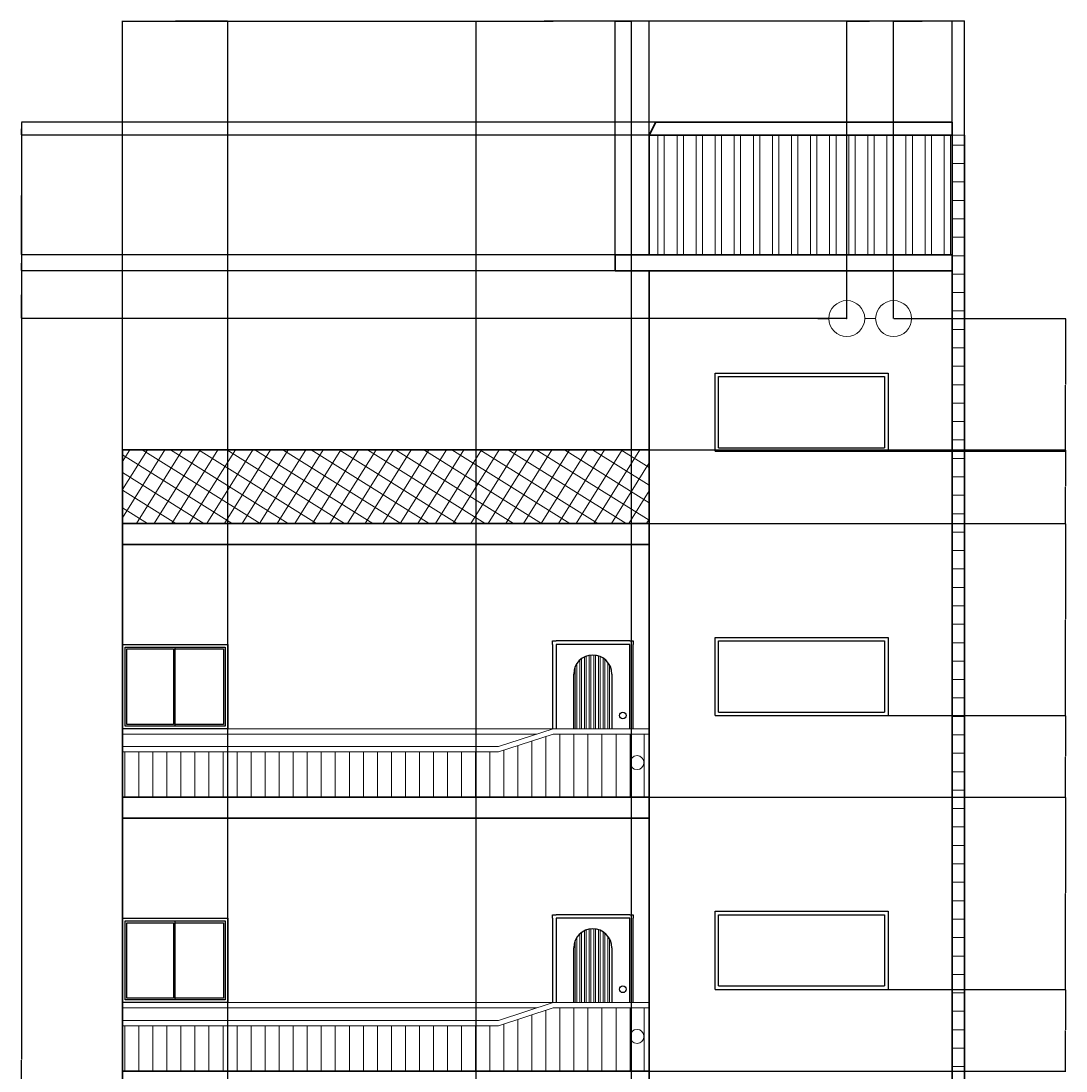
# Model space of a CAD drawing. Units: inches. Extents: x 373 to 969, y 157 to 1341.
# Tile 3 of 3: x 373 to 968, y 743 to 1341. Entities that reach past the tile are written whole.
import ezdxf

# ---------------------------------------------------------------- set-up
doc = ezdxf.new("R2010")
doc.units = ezdxf.units.IN
doc.header["$MEASUREMENT"] = 0
for name, color, linetype, lineweight in [('A-ANNO-DIMS', 2, 'Continuous', 18), ('A-DOOR', 3, 'Continuous', 25), ('A-DOOR-PATT', 8, 'Continuous', 13), ('A-ELEV-TRIM', 9, 'Continuous', 18), ('A-FLOR', 7, 'Continuous', 30), ('A-FLOR-HRAL', 4, 'Continuous', 18), ('A-FLOR-HRAL-PATT', 8, 'Continuous', 13), ('A-GLAZ', 4, 'Continuous', 25), ('A-ROOF', 7, 'Continuous', 30), ('A-WALL', 7, 'Continuous', 35), ('A-WALL-PATT', 8, 'Continuous', 13)]:
    doc.layers.add(name, color=color, linetype=linetype, lineweight=lineweight)
doc.styles.get("Standard").update_dxf_attribs({"font": 'arial.ttf'})
doc.dimstyles.get("Standard").update_dxf_attribs({"dimtxt": 0.18, "dimasz": 0.18, "dimexe": 0.18, "dimexo": 0.0625, "dimgap": 0.09, "dimtad": 0, "dimtih": 1, "dimtoh": 1, "dimdec": 4, "dimzin": 0, "dimdsep": 46, "dimlunit": 4, "dimtxsty": 'Standard', "dimcen": 0.09, "dimadec": 0, "dimazin": 0, "dimtfac": 1, "dimtdec": 4, "dimtofl": 0, "dimtmove": 0, "dimatfit": 3, "dimfxl": 1, "dimtolj": 1, "dimtzin": 0, "dimarcsym": 0})

# ---------------------------------------------------------------- blocks, each defined once
blk = doc.blocks.new('*U2')
for p, q in [((1.5, 1.5), (1.5, 46.5)), ((1.5, 46.5), (30, 46.5)), ((30, 1.5), (30, 46.5)), ((30, 46.5), (58.5, 46.5)), ((58.5, 46.5), (58.5, 1.5)), ((30, 1.5), (1.5, 1.5)), ((58.5, 1.5), (30, 1.5))]:
    blk.add_line(p, q)
blk.add_lwpolyline([(0, 0), (0, 48), (60, 48), (60, 0)], close=True)
for points in [[(29, 45.5), (29, 2.5), (2.5, 2.5), (2.5, 45.5), (29, 45.5)], [(30, 45.5), (57.5, 45.5), (57.5, 2.5), (30, 2.5)]]:
    blk.add_lwpolyline(points)
blk = doc.blocks.new('DOOR-ARCH-PANEL-ELEV')
for p, q in [((0, 48), (0, 50)), ((0, 50), (2, 50)), ((0, 48), (0, 0)), ((44, 50), (2, 50)), ((44, 48), (2, 48)), ((2, 48), (2, 0)), ((44, 50), (46, 50)), ((44, 0), (44, 48)), ((46, 50), (46, 48)), ((46, 0), (46, 48))]:
    blk.add_line(p, q)
for points in [[(12.07, 0), (12.07, 31.15)], [(33.78, 31.15), (33.78, 0)]]:
    blk.add_lwpolyline(points)
blk.add_circle((40.06, 7.56), 1.92)
blk.add_arc((22.93, 31.15), 10.86, 0, 180)
blk = doc.blocks.new('RAIL-BALCONY-SLOPED-ELEV')
for p, q in [((245.4, 23.26), (0, 23.26)), ((236.25, 20.26), (0, 20.26)), ((245.4, 23.26), (214.4, 13.09)), ((245.4, 20.26), (214.4, 10.09)), ((300.23, 23.26), (245.4, 23.26)), ((300.23, 20.26), (245.4, 20.26)), ((214.4, 13.09), (0, 13.09)), ((214.4, 10.09), (0, 10.09))]:
    blk.add_line(p, q)
blk.add_circle((293.27, 3.97), 3.97)
blk = doc.blocks.new('WIN-FIXED-FRAME-ELEV')
for p, q in [((0, 0), (98.59, 0)), ((2, 2), (96.59, 2))]:
    blk.add_line(p, q)
for points in [[(0, 0), (0, 44.5), (98.59, 44.5), (98.59, 0)], [(2, 2), (2, 42.5), (96.59, 42.5), (96.59, 2)]]:
    blk.add_lwpolyline(points)
blk = doc.blocks.new('*D20')
at = {"layer": 'A-ANNO-DIMS', "color": 0, "lineweight": -2, "transparency": 16777216}
for p, q in [((867.13, 789.48), (968.33, 789.48)), ((968.15, 789.3), (968.15, 766.42)), ((968.15, 743.16), (968.15, 766.05)), ((731, 742.98), (968.33, 742.98))]:
    blk.add_line(p, q, dxfattribs=at)
at = {"layer": 'A-ANNO-DIMS', "color": 0, "transparency": 16777216}
for points in [[(968.12, 789.3), (968.18, 789.3), (968.15, 789.48)], [(968.12, 743.16), (968.18, 743.16), (968.15, 742.98)]]:
    blk.add_solid(points, dxfattribs=at)
at = {"layer": 'Defpoints', "color": 0, "transparency": 16777216}
for p in [(867.07, 789.48), (968.15, 789.48), (730.93, 742.98)]:
    blk.add_point(p, dxfattribs=at)
at = {"layer": 'A-ANNO-DIMS', "color": 0, "transparency": 16777216, "insert": (968.15, 766.23), "char_height": 0.18, "attachment_point": 5}
blk.add_mtext('\\A1;46.5', dxfattribs=at)
blk = doc.blocks.new('*D21')
at = {"layer": 'A-ANNO-DIMS', "color": 0, "lineweight": -2, "transparency": 16777216}
for p, q in [((731, 898.98), (968.33, 898.98)), ((968.15, 898.8), (968.15, 844.42)), ((968.15, 789.66), (968.15, 844.05)), ((867.13, 789.48), (968.33, 789.48))]:
    blk.add_line(p, q, dxfattribs=at)
at = {"layer": 'A-ANNO-DIMS', "color": 0, "transparency": 16777216}
for points in [[(968.12, 898.8), (968.18, 898.8), (968.15, 898.98)], [(968.12, 789.66), (968.18, 789.66), (968.15, 789.48)]]:
    blk.add_solid(points, dxfattribs=at)
at = {"layer": 'Defpoints', "color": 0, "transparency": 16777216}
for p in [(730.93, 898.98), (968.15, 898.98), (867.07, 789.48)]:
    blk.add_point(p, dxfattribs=at)
at = {"layer": 'A-ANNO-DIMS', "color": 0, "transparency": 16777216, "insert": (968.15, 844.23), "char_height": 0.18, "attachment_point": 5}
blk.add_mtext('\\A1;109.5', dxfattribs=at)
blk = doc.blocks.new('*D22')
at = {"layer": 'A-ANNO-DIMS', "color": 0, "lineweight": -2, "transparency": 16777216}
for p, q in [((867.13, 945.48), (968.33, 945.48)), ((968.15, 945.3), (968.15, 922.42)), ((968.15, 899.16), (968.15, 922.05)), ((731, 898.98), (968.33, 898.98))]:
    blk.add_line(p, q, dxfattribs=at)
at = {"layer": 'A-ANNO-DIMS', "color": 0, "transparency": 16777216}
for points in [[(968.12, 945.3), (968.18, 945.3), (968.15, 945.48)], [(968.12, 899.16), (968.18, 899.16), (968.15, 898.98)]]:
    blk.add_solid(points, dxfattribs=at)
at = {"layer": 'Defpoints', "color": 0, "transparency": 16777216}
for p in [(867.07, 945.48), (968.15, 945.48), (730.93, 898.98)]:
    blk.add_point(p, dxfattribs=at)
at = {"layer": 'A-ANNO-DIMS', "color": 0, "transparency": 16777216, "insert": (968.15, 922.23), "char_height": 0.18, "attachment_point": 5}
blk.add_mtext('\\A1;46.5', dxfattribs=at)
blk = doc.blocks.new('*D23')
at = {"layer": 'A-ANNO-DIMS', "color": 0, "lineweight": -2, "transparency": 16777216}
for p, q in [((731, 1054.98), (968.33, 1054.98)), ((968.15, 1054.8), (968.15, 1000.42)), ((968.15, 945.66), (968.15, 1000.05)), ((867.13, 945.48), (968.33, 945.48))]:
    blk.add_line(p, q, dxfattribs=at)
at = {"layer": 'A-ANNO-DIMS', "color": 0, "transparency": 16777216}
for points in [[(968.12, 1054.8), (968.18, 1054.8), (968.15, 1054.98)], [(968.12, 945.66), (968.18, 945.66), (968.15, 945.48)]]:
    blk.add_solid(points, dxfattribs=at)
at = {"layer": 'Defpoints', "color": 0, "transparency": 16777216}
for p in [(730.93, 1054.98), (968.15, 1054.98), (867.07, 945.48)]:
    blk.add_point(p, dxfattribs=at)
at = {"layer": 'A-ANNO-DIMS', "color": 0, "transparency": 16777216, "insert": (968.15, 1000.23), "char_height": 0.18, "attachment_point": 5}
blk.add_mtext('\\A1;109.5', dxfattribs=at)
blk = doc.blocks.new('*D24')
at = {"layer": 'A-ANNO-DIMS', "color": 0, "lineweight": -2, "transparency": 16777216}
for p, q in [((731, 1096.98), (968.33, 1096.98)), ((968.15, 1096.8), (968.15, 1076.16)), ((968.15, 1055.16), (968.15, 1075.8)), ((731, 1054.98), (968.33, 1054.98))]:
    blk.add_line(p, q, dxfattribs=at)
at = {"layer": 'A-ANNO-DIMS', "color": 0, "transparency": 16777216}
for points in [[(968.12, 1096.8), (968.18, 1096.8), (968.15, 1096.98)], [(968.12, 1055.16), (968.18, 1055.16), (968.15, 1054.98)]]:
    blk.add_solid(points, dxfattribs=at)
at = {"layer": 'Defpoints', "color": 0, "transparency": 16777216}
for p in [(730.93, 1096.98), (968.15, 1096.98), (730.93, 1054.98)]:
    blk.add_point(p, dxfattribs=at)
at = {"layer": 'A-ANNO-DIMS', "color": 0, "transparency": 16777216, "insert": (968.15, 1075.98), "char_height": 0.18, "attachment_point": 5}
blk.add_mtext('\\A1;42', dxfattribs=at)
blk = doc.blocks.new('*D29')
at = {"layer": 'A-ANNO-DIMS', "color": 0, "lineweight": -2, "transparency": 16777216}
for p, q in [((430.7, 518.05), (430.7, 1341.24)), ((430.88, 1341.06), (460.48, 1341.06)), ((490.52, 1341.06), (460.92, 1341.06)), ((490.7, 518.05), (490.7, 1341.24))]:
    blk.add_line(p, q, dxfattribs=at)
at = {"layer": 'A-ANNO-DIMS', "color": 0, "transparency": 16777216}
for points in [[(430.88, 1341.09), (430.88, 1341.03), (430.7, 1341.06)], [(490.52, 1341.09), (490.52, 1341.03), (490.7, 1341.06)]]:
    blk.add_solid(points, dxfattribs=at)
at = {"layer": 'Defpoints', "color": 0, "transparency": 16777216}
for p in [(490.7, 1341.06), (430.7, 517.98), (490.7, 517.98)]:
    blk.add_point(p, dxfattribs=at)
at = {"layer": 'A-ANNO-DIMS', "color": 0, "transparency": 16777216, "insert": (460.7, 1341.06), "char_height": 0.18, "attachment_point": 5}
blk.add_mtext('\\A1;60', dxfattribs=at)
blk = doc.blocks.new('*D42')
at = {"layer": 'A-ANNO-DIMS', "color": 0, "lineweight": -2, "transparency": 16777216}
for p, q in [((632.3, 362.67), (632.3, 1341.24)), ((632.48, 1341.06), (676.2, 1341.06)), ((720.7, 1341.06), (676.98, 1341.06)), ((720.88, 362.67), (720.88, 1341.24))]:
    blk.add_line(p, q, dxfattribs=at)
at = {"layer": 'A-ANNO-DIMS', "color": 0, "transparency": 16777216}
for points in [[(632.48, 1341.09), (632.48, 1341.03), (632.3, 1341.06)], [(720.7, 1341.09), (720.7, 1341.03), (720.88, 1341.06)]]:
    blk.add_solid(points, dxfattribs=at)
at = {"layer": 'Defpoints', "color": 0, "transparency": 16777216}
for p in [(720.88, 1341.06), (632.3, 362.6), (720.88, 362.6)]:
    blk.add_point(p, dxfattribs=at)
at = {"layer": 'A-ANNO-DIMS', "color": 0, "transparency": 16777216, "insert": (676.59, 1341.06), "char_height": 0.18, "attachment_point": 5}
blk.add_mtext('\\A1;88.58', dxfattribs=at)
blk = doc.blocks.new('*D46')
at = {"layer": 'A-ANNO-DIMS', "color": 0, "lineweight": -2, "transparency": 16777216}
for p, q in [((843.49, 1171.75), (843.49, 1341.24)), ((843.67, 1341.06), (856.39, 1341.06)), ((870.03, 1341.06), (857.32, 1341.06)), ((870.21, 1171.75), (870.21, 1341.24))]:
    blk.add_line(p, q, dxfattribs=at)
at = {"layer": 'A-ANNO-DIMS', "color": 0, "transparency": 16777216}
for points in [[(843.67, 1341.09), (843.67, 1341.03), (843.49, 1341.06)], [(870.03, 1341.09), (870.03, 1341.03), (870.21, 1341.06)]]:
    blk.add_solid(points, dxfattribs=at)
at = {"layer": 'Defpoints', "color": 0, "transparency": 16777216}
for p in [(870.21, 1341.06), (843.49, 1171.69), (870.21, 1171.69)]:
    blk.add_point(p, dxfattribs=at)
at = {"layer": 'A-ANNO-DIMS', "color": 0, "transparency": 16777216, "insert": (856.85, 1341.06), "char_height": 0.18, "attachment_point": 5}
blk.add_mtext('\\A1;26.724', dxfattribs=at)
blk = doc.blocks.new('*D47')
at = {"layer": 'A-ANNO-DIMS', "color": 0, "lineweight": -2, "transparency": 16777216}
for p, q in [((870.21, 1171.75), (870.21, 1341.24)), ((870.39, 1341.06), (886.42, 1341.06)), ((903.37, 1341.06), (887.35, 1341.06)), ((903.55, 1171.75), (903.55, 1341.24))]:
    blk.add_line(p, q, dxfattribs=at)
at = {"layer": 'A-ANNO-DIMS', "color": 0, "transparency": 16777216}
for points in [[(870.39, 1341.09), (870.39, 1341.03), (870.21, 1341.06)], [(903.37, 1341.09), (903.37, 1341.03), (903.55, 1341.06)]]:
    blk.add_solid(points, dxfattribs=at)
at = {"layer": 'Defpoints', "color": 0, "transparency": 16777216}
for p in [(903.55, 1341.06), (870.21, 1171.69), (903.55, 1171.69)]:
    blk.add_point(p, dxfattribs=at)
at = {"layer": 'A-ANNO-DIMS', "color": 0, "transparency": 16777216, "insert": (886.88, 1341.06), "char_height": 0.18, "attachment_point": 5}
blk.add_mtext('\\A1;33.335', dxfattribs=at)
blk = doc.blocks.new('*D48')
at = {"layer": 'A-ANNO-DIMS', "color": 0, "lineweight": -2, "transparency": 16777216}
for p, q in [((870.28, 1171.69), (968.33, 1171.69)), ((968.15, 1171.51), (968.15, 1134.07)), ((968.15, 1096.27), (968.15, 1133.71)), ((867.13, 1096.09), (968.33, 1096.09))]:
    blk.add_line(p, q, dxfattribs=at)
at = {"layer": 'A-ANNO-DIMS', "color": 0, "transparency": 16777216}
for points in [[(968.12, 1171.51), (968.18, 1171.51), (968.15, 1171.69)], [(968.12, 1096.27), (968.18, 1096.27), (968.15, 1096.09)]]:
    blk.add_solid(points, dxfattribs=at)
at = {"layer": 'Defpoints', "color": 0, "transparency": 16777216}
for p in [(870.21, 1171.69), (867.07, 1096.09), (968.15, 1096.09)]:
    blk.add_point(p, dxfattribs=at)
at = {"layer": 'A-ANNO-DIMS', "color": 0, "transparency": 16777216, "insert": (968.15, 1133.89), "char_height": 0.18, "attachment_point": 5}
blk.add_mtext('\\A1;75.59', dxfattribs=at)
blk = doc.blocks.new('*D49')
at = {"layer": 'A-ANNO-DIMS', "color": 0, "lineweight": -2, "transparency": 16777216}
for p, q in [((730.87, 1198.98), (373.07, 1198.98)), ((373.25, 1198.8), (373.25, 1185.52)), ((373.25, 1171.87), (373.25, 1185.15)), ((843.43, 1171.69), (373.07, 1171.69))]:
    blk.add_line(p, q, dxfattribs=at)
at = {"layer": 'A-ANNO-DIMS', "color": 0, "transparency": 16777216}
for points in [[(373.22, 1198.8), (373.28, 1198.8), (373.25, 1198.98)], [(373.22, 1171.87), (373.28, 1171.87), (373.25, 1171.69)]]:
    blk.add_solid(points, dxfattribs=at)
at = {"layer": 'Defpoints', "color": 0, "transparency": 16777216}
for p in [(373.25, 1198.98), (730.93, 1198.98), (843.49, 1171.69)]:
    blk.add_point(p, dxfattribs=at)
at = {"layer": 'A-ANNO-DIMS', "color": 0, "transparency": 16777216, "insert": (373.25, 1185.34), "char_height": 0.18, "attachment_point": 5}
blk.add_mtext('\\A1;27.3', dxfattribs=at)
blk = doc.blocks.new('*D50')
at = {"layer": 'A-ANNO-DIMS', "color": 0, "lineweight": -2, "transparency": 16777216}
for p, q in [((711.52, 1207.98), (373.07, 1207.98)), ((373.25, 1207.8), (373.25, 1203.67)), ((373.25, 1199.16), (373.25, 1203.3)), ((711.52, 1198.98), (373.07, 1198.98))]:
    blk.add_line(p, q, dxfattribs=at)
at = {"layer": 'A-ANNO-DIMS', "color": 0, "transparency": 16777216}
for points in [[(373.22, 1207.8), (373.28, 1207.8), (373.25, 1207.98)], [(373.22, 1199.16), (373.28, 1199.16), (373.25, 1198.98)]]:
    blk.add_solid(points, dxfattribs=at)
at = {"layer": 'Defpoints', "color": 0, "transparency": 16777216}
for p in [(373.25, 1207.98), (711.59, 1207.98), (711.59, 1198.98)]:
    blk.add_point(p, dxfattribs=at)
at = {"layer": 'A-ANNO-DIMS', "color": 0, "transparency": 16777216, "insert": (373.25, 1203.48), "char_height": 0.18, "attachment_point": 5}
blk.add_mtext('\\A1;9', dxfattribs=at)
blk = doc.blocks.new('*D51')
at = {"layer": 'A-ANNO-DIMS', "color": 0, "lineweight": -2, "transparency": 16777216}
for p, q in [((730.87, 1276.18), (373.07, 1276.18)), ((373.25, 1276), (373.25, 1242.26)), ((373.25, 1208.16), (373.25, 1241.9)), ((730.87, 1207.98), (373.07, 1207.98))]:
    blk.add_line(p, q, dxfattribs=at)
at = {"layer": 'A-ANNO-DIMS', "color": 0, "transparency": 16777216}
for points in [[(373.22, 1276), (373.28, 1276), (373.25, 1276.18)], [(373.22, 1208.16), (373.28, 1208.16), (373.25, 1207.98)]]:
    blk.add_solid(points, dxfattribs=at)
at = {"layer": 'Defpoints', "color": 0, "transparency": 16777216}
for p in [(373.25, 1276.18), (730.93, 1276.18), (730.93, 1207.98)]:
    blk.add_point(p, dxfattribs=at)
at = {"layer": 'A-ANNO-DIMS', "color": 0, "transparency": 16777216, "insert": (373.25, 1242.08), "char_height": 0.18, "attachment_point": 5}
blk.add_mtext('\\A1;68.19', dxfattribs=at)
blk = doc.blocks.new('*D52')
at = {"layer": 'A-ANNO-DIMS', "color": 0, "lineweight": -2, "transparency": 16777216}
for p, q in [((734.58, 1283.61), (373.07, 1283.61)), ((373.25, 1283.43), (373.25, 1280.07)), ((730.87, 1276.18), (373.07, 1276.18)), ((373.25, 1276.36), (373.25, 1279.71))]:
    blk.add_line(p, q, dxfattribs=at)
at = {"layer": 'A-ANNO-DIMS', "color": 0, "transparency": 16777216}
for points in [[(373.22, 1283.43), (373.28, 1283.43), (373.25, 1283.61)], [(373.22, 1276.36), (373.28, 1276.36), (373.25, 1276.18)]]:
    blk.add_solid(points, dxfattribs=at)
at = {"layer": 'Defpoints', "color": 0, "transparency": 16777216}
for p in [(373.25, 1283.61), (734.64, 1283.61), (730.93, 1276.18)]:
    blk.add_point(p, dxfattribs=at)
at = {"layer": 'A-ANNO-DIMS', "color": 0, "transparency": 16777216, "insert": (373.25, 1279.89), "char_height": 0.18, "attachment_point": 5}
blk.add_mtext('\\A1;7.431', dxfattribs=at)
blk = doc.blocks.new('*D53')
at = {"layer": 'A-ANNO-DIMS', "color": 0, "lineweight": -2, "transparency": 16777216}
for p, q in [((711.59, 1208.05), (711.59, 1341.24)), ((711.77, 1341.06), (720.81, 1341.06)), ((730.75, 1341.06), (721.72, 1341.06)), ((730.93, 1208.05), (730.93, 1341.24))]:
    blk.add_line(p, q, dxfattribs=at)
at = {"layer": 'A-ANNO-DIMS', "color": 0, "transparency": 16777216}
for points in [[(711.77, 1341.09), (711.77, 1341.03), (711.59, 1341.06)], [(730.75, 1341.09), (730.75, 1341.03), (730.93, 1341.06)]]:
    blk.add_solid(points, dxfattribs=at)
at = {"layer": 'Defpoints', "color": 0, "transparency": 16777216}
for p in [(730.93, 1341.06), (711.59, 1207.98), (730.93, 1207.98)]:
    blk.add_point(p, dxfattribs=at)
at = {"layer": 'A-ANNO-DIMS', "color": 0, "transparency": 16777216, "insert": (721.26, 1341.06), "char_height": 0.18, "attachment_point": 5}
blk.add_mtext('\\A1;19.346', dxfattribs=at)
blk = doc.blocks.new('*D54')
at = {"layer": 'A-ANNO-DIMS', "color": 0, "lineweight": -2, "transparency": 16777216}
for p, q in [((430.7, 1097.05), (430.7, 1341.24)), ((430.88, 1341.06), (670.41, 1341.06)), ((910.52, 1341.06), (670.99, 1341.06)), ((910.7, 1276.24), (910.7, 1341.24))]:
    blk.add_line(p, q, dxfattribs=at)
at = {"layer": 'A-ANNO-DIMS', "color": 0, "transparency": 16777216}
for points in [[(430.88, 1341.09), (430.88, 1341.03), (430.7, 1341.06)], [(910.52, 1341.09), (910.52, 1341.03), (910.7, 1341.06)]]:
    blk.add_solid(points, dxfattribs=at)
at = {"layer": 'Defpoints', "color": 0, "transparency": 16777216}
for p in [(910.7, 1341.06), (910.7, 1276.18), (430.7, 1096.98)]:
    blk.add_point(p, dxfattribs=at)
at = {"layer": 'A-ANNO-DIMS', "color": 0, "transparency": 16777216, "insert": (670.7, 1341.06), "char_height": 0.18, "attachment_point": 5}
blk.add_mtext('\\A1;480', dxfattribs=at)
blk = doc.blocks.new('*D55')
at = {"layer": 'A-ANNO-DIMS', "color": 0, "lineweight": -2, "transparency": 16777216}
for p, q in [((734.58, 1283.61), (373.07, 1283.61)), ((373.25, 1283.43), (373.25, 749.48)), ((373.25, 215.16), (373.25, 749.11)), ((430.64, 214.98), (373.07, 214.98))]:
    blk.add_line(p, q, dxfattribs=at)
at = {"layer": 'A-ANNO-DIMS', "color": 0, "transparency": 16777216}
for points in [[(373.22, 1283.43), (373.28, 1283.43), (373.25, 1283.61)], [(373.22, 215.16), (373.28, 215.16), (373.25, 214.98)]]:
    blk.add_solid(points, dxfattribs=at)
at = {"layer": 'Defpoints', "color": 0, "transparency": 16777216}
for p in [(373.25, 1283.61), (734.64, 1283.61), (430.7, 214.98)]:
    blk.add_point(p, dxfattribs=at)
at = {"layer": 'A-ANNO-DIMS', "color": 0, "transparency": 16777216, "insert": (373.25, 749.3), "char_height": 0.18, "attachment_point": 5}
blk.add_mtext('\\A1;1068.6', dxfattribs=at)
blk = doc.blocks.new('*D61')
at = {"layer": 'A-ANNO-DIMS', "color": 0, "lineweight": -2, "transparency": 16777216}
for p, q in [((827.1, 1171.71), (833.06, 1171.7)), ((843.4, 1171.69), (843.58, 1171.69)), ((843.49, 1171.6), (843.49, 1171.78))]:
    blk.add_line(p, q, dxfattribs=at)
at = {"layer": 'A-ANNO-DIMS', "color": 0, "transparency": 16777216}
blk.add_solid([(833.06, 1171.73), (833.06, 1171.67), (833.24, 1171.7)], dxfattribs=at)
at = {"layer": 'Defpoints', "color": 0, "transparency": 16777216}
for p in [(833.24, 1171.7), (853.73, 1171.67)]:
    blk.add_point(p, dxfattribs=at)
at = {"layer": 'A-ANNO-DIMS', "color": 0, "transparency": 16777216, "insert": (826.42, 1171.71), "char_height": 0.18, "attachment_point": 5}
blk.add_mtext('\\A1;2X ∅20.49', dxfattribs=at)

msp = doc.modelspace()

# ---------------------------------------------------------------- hatches: boundary and pattern name
at = {"layer": 'A-DOOR-PATT'}
h = msp.add_hatch(dxfattribs=at)
h.set_pattern_fill('ANSI32', color=256, scale=7.1, angle=225)
h.set_pattern_definition([(270, (2e-13, 468), (2.6625, -4e-16), []), (270, (-0.8875, 467.1125), (2.6625, -4e-16), [])])
h.paths.add_polyline_path([(709.6057, 969.1302, 1), (687.8953, 969.1302), (687.8953, 937.9843), (709.6057, 937.9843)])
h = msp.add_hatch(dxfattribs=at)
h.set_pattern_fill('ANSI32', color=256, scale=7.1, angle=225)
h.set_pattern_definition([(270, (1e-13, 312), (2.6625, -4e-16), []), (270, (-0.8875, 311.1125), (2.6625, -4e-16), [])])
h.paths.add_polyline_path([(709.6057, 813.1302, 1), (687.8953, 813.1302), (687.8953, 781.9843), (709.6057, 781.9843)])
at = {"layer": 'A-FLOR-HRAL-PATT'}
h = msp.add_hatch(dxfattribs=at)
h.set_pattern_fill('ANSI31', color=256, scale=64, angle=225)
h.set_pattern_definition([(270, (2e-13, 468), (8, -9e-16), [])])
h.paths.add_polyline_path([(730.9335, 934.9843), (676.0953, 934.9843), (645.0983, 924.8114), (430.6998, 924.8114), (430.6998, 898.9843), (730.9335, 898.9843)])
h = msp.add_hatch(dxfattribs=at)
h.set_pattern_fill('ANSI31', color=256, scale=64, angle=225)
h.set_pattern_definition([(270, (1e-13, 312), (8, -9e-16), [])])
h.paths.add_polyline_path([(730.9335, 778.9843), (676.0953, 778.9843), (645.0983, 768.8114), (430.6998, 768.8114), (430.6998, 742.9843), (730.9335, 742.9843)])
at = {"layer": 'A-WALL-PATT'}
h = msp.add_hatch(dxfattribs=at)
h.set_pattern_fill('ANSI32', color=256, scale=29, angle=225)
h.paths.add_polyline_path([(903.5487, 1276.1757), (730.9335, 1276.1757), (730.9335, 1207.9843), (903.5487, 1207.9843)])
h = msp.add_hatch(dxfattribs=at)
h.set_pattern_fill('ANSI31', color=256, scale=84, angle=315)
h.paths.add_polyline_path([(910.6998, 1276.1757), (903.5487, 1276.1757), (903.5487, 430.9843), (910.6998, 430.9843)])
h = msp.add_hatch(dxfattribs=at)
h.set_pattern_fill('ANSI37', color=256, scale=68, angle=193)
h.paths.add_polyline_path([(730.9335, 1096.9843), (430.6998, 1096.9843), (430.6998, 1054.9843), (730.9335, 1054.9843)])

# ---------------------------------------------------------------- linework, layer by layer
at = {"layer": 'A-ELEV-TRIM'}
for p, q in [((903.5487, 1276.1757), (910.6998, 1276.1757)), ((730.9335, 1171.6862), (833.2445, 1171.6862)), ((853.7343, 1171.6862), (859.969, 1171.6862)), ((880.4588, 1171.6862), (903.5487, 1171.6862))]:
    msp.add_line(p, q, dxfattribs=at)
for centre in [(843.4894, 1171.6862), (870.2139, 1171.6862)]:
    msp.add_circle(centre, 10.2449, dxfattribs=at)
at = {"layer": 'A-FLOR'}
for p, q in [((430.6998, 1042.9843), (430.6998, 1054.9843)), ((430.6998, 1054.9843), (730.9335, 1054.9843)), ((430.6998, 1042.9843), (730.9335, 1042.9843)), ((430.6998, 886.9843), (430.6998, 898.9843)), ((430.6998, 898.9843), (730.9335, 898.9843)), ((430.6998, 886.9843), (730.9335, 886.9843)), ((430.6998, 730.9843), (430.6998, 742.9843)), ((430.6998, 742.9843), (730.9335, 742.9843))]:
    msp.add_line(p, q, dxfattribs=at)
at = {"layer": 'A-ROOF'}
for p, q in [((730.9335, 1276.1757), (734.6424, 1283.6064)), ((734.6424, 1283.6064), (903.5487, 1283.6064)), ((730.9335, 1207.9843), (730.9335, 1276.1757)), ((903.5487, 1276.1757), (730.9335, 1276.1757)), ((730.9335, 1207.9843), (711.587, 1207.9843)), ((711.587, 1207.9843), (711.587, 1198.9843)), ((730.9335, 1207.9843), (903.5487, 1207.9843)), ((711.587, 1198.9843), (730.9335, 1198.9843)), ((730.9335, 1054.9843), (730.9335, 1198.9843)), ((730.9335, 1198.9843), (903.5487, 1198.9843)), ((430.6998, 1054.9843), (430.6998, 1096.9843)), ((430.6998, 1096.9843), (730.9335, 1096.9843))]:
    msp.add_line(p, q, dxfattribs=at)
at = {"layer": 'A-WALL'}
for p, q in [((903.5487, 430.9843), (903.5487, 1283.6064)), ((730.9335, 856.4498), (730.9335, 1198.9843)), ((430.6998, 898.9843), (430.6998, 1042.9843)), ((430.6998, 742.9843), (430.6998, 886.9843)), ((730.9335, 587.7283), (730.9335, 856.4498))]:
    msp.add_line(p, q, dxfattribs=at)
msp.add_lwpolyline([(430.6998, 430.9843), (910.6998, 430.9843), (910.6998, 1276.1757)], dxfattribs=at)

# ---------------------------------------------------------------- block references
at = {"layer": 'A-DOOR'}
for p in [(675.824, 937.984), (675.824, 781.984)]:
    msp.add_blockref('DOOR-ARCH-PANEL-ELEV', p, dxfattribs=at)
at = {"layer": 'A-FLOR-HRAL'}
for p in [(430.7, 914.722), (430.7, 758.722)]:
    msp.add_blockref('RAIL-BALCONY-SLOPED-ELEV', p, dxfattribs=at)
at = {"layer": 'A-GLAZ'}
for name, p in [('WIN-FIXED-FRAME-ELEV', (768.476, 1096.0941)), ('WIN-FIXED-FRAME-ELEV', (768.476, 945.484)), ('*U2', (430.6998, 937.9843)), ('WIN-FIXED-FRAME-ELEV', (768.476, 789.484)), ('*U2', (430.6998, 781.9843))]:
    msp.add_blockref(name, p, dxfattribs=at)

# ---------------------------------------------------------------- dimensions: what is measured, and where the dimension line sits
at = {"layer": 'A-ANNO-DIMS'}
for base, p1, p2, override, picture, middle in [((490.6998, 1341.0564), (430.6998, 517.9843), (490.6998, 517.9843), {"dimdec": 0, "dimlfac": 1, "dimrnd": 0, "dimzin": 0, "dimdsep": 46, "dimlunit": 2}, '*D29', (460.6998, 1341.0564)), ((910.6998, 1341.0564), (430.6998, 1096.9843), (910.6998, 1276.1757), {"dimdec": 0, "dimlfac": 1, "dimrnd": 0, "dimzin": 0, "dimdsep": 46, "dimlunit": 2}, '*D54', (670.6998, 1341.0564)), ((720.8808, 1341.0564), (632.3006, 362.6044), (720.8808, 362.6044), {"dimdec": 2, "dimlfac": 1, "dimrnd": 0, "dimzin": 0, "dimdsep": 46, "dimlunit": 2}, '*D42', (676.5907, 1341.0564)), ((730.93345, 1341.05642), (711.58705, 1207.9843), (730.93345, 1207.9843), {"dimdec": 3, "dimlfac": 1, "dimrnd": 0, "dimzin": 0, "dimdsep": 46, "dimlunit": 2}, '*D53', (721.26025, 1341.05642)), ((870.21388, 1341.05642), (843.4894, 1171.6862), (870.21388, 1171.6862), {"dimdec": 3, "dimlfac": 1, "dimrnd": 0, "dimzin": 0, "dimdsep": 46, "dimlunit": 2}, '*D46', (856.85164, 1341.05642)), ((903.5487, 1341.0564), (870.2139, 1171.6862), (903.5487, 1171.6862), {"dimdec": 3, "dimlfac": 1, "dimrnd": 0, "dimzin": 0, "dimdsep": 46, "dimlunit": 2}, '*D47', (886.8813, 1341.0564))]:
    dim = msp.add_linear_dim(base=base, p1=p1, p2=p2, dimstyle='Standard', override=override, dxfattribs=at)
    dim.commit()
    dim.dimension.update_dxf_attribs({"geometry": picture, "text_midpoint": middle})
for base, p1, p2, override, picture, middle in [((373.2498, 1283.6064), (430.6998, 214.9843), (734.6424, 1283.6064), {"dimdec": 1, "dimlfac": 1, "dimrnd": 0, "dimzin": 0, "dimdsep": 46, "dimlunit": 2}, '*D55', (373.2498, 749.2954)), ((373.2498, 1283.6064), (730.9335, 1276.1757), (734.6424, 1283.6064), {"dimdec": 3, "dimlfac": 1, "dimrnd": 0, "dimzin": 0, "dimdsep": 46, "dimlunit": 2}, '*D52', (373.2498, 1279.8911)), ((373.2498, 1276.1757), (730.9335, 1207.9843), (730.9335, 1276.1757), {"dimdec": 2, "dimlfac": 1, "dimrnd": 0, "dimzin": 0, "dimdsep": 46, "dimlunit": 2}, '*D51', (373.2498, 1242.08)), ((373.2498, 1207.9843), (711.587, 1198.9843), (711.587, 1207.9843), {"dimdec": 0, "dimlfac": 1, "dimrnd": 0, "dimzin": 0, "dimdsep": 46, "dimlunit": 2}, '*D50', (373.2498, 1203.4843)), ((373.2498, 1198.9843), (843.4894, 1171.6862), (730.9335, 1198.9843), {"dimdec": 1, "dimlfac": 1, "dimrnd": 0, "dimzin": 0, "dimdsep": 46, "dimlunit": 2}, '*D49', (373.2498, 1185.3353)), ((968.1498, 1096.0944), (870.2139, 1171.6862), (867.0679, 1096.0944), {"dimdec": 2, "dimlfac": 1, "dimrnd": 0, "dimzin": 0, "dimdsep": 46, "dimlunit": 2}, '*D48', (968.1498, 1133.8903)), ((968.1498, 1096.9843), (730.9335, 1054.9843), (730.9335, 1096.9843), {"dimdec": 0, "dimlfac": 1, "dimrnd": 0, "dimzin": 0, "dimdsep": 46, "dimlunit": 2}, '*D24', (968.1498, 1075.9843)), ((968.1498, 1054.9843), (867.0679, 945.4843), (730.9335, 1054.9843), {"dimdec": 1, "dimlfac": 1, "dimrnd": 0, "dimzin": 0, "dimdsep": 46, "dimlunit": 2}, '*D23', (968.1498, 1000.2343)), ((968.1498, 945.4843), (730.9335, 898.9843), (867.0679, 945.4843), {"dimdec": 1, "dimlfac": 1, "dimrnd": 0, "dimzin": 0, "dimdsep": 46, "dimlunit": 2}, '*D22', (968.1498, 922.2343)), ((968.1498, 898.9843), (867.0679, 789.4843), (730.9335, 898.9843), {"dimdec": 1, "dimlfac": 1, "dimrnd": 0, "dimzin": 0, "dimdsep": 46, "dimlunit": 2}, '*D21', (968.1498, 844.2343)), ((968.1498, 789.4843), (730.9335, 742.9843), (867.0679, 789.4843), {"dimdec": 1, "dimlfac": 1, "dimrnd": 0, "dimzin": 0, "dimdsep": 46, "dimlunit": 2}, '*D20', (968.1498, 766.2343))]:
    dim = msp.add_linear_dim(base=base, p1=p1, p2=p2, angle=90, dimstyle='Standard', override=override, dxfattribs=at)
    dim.commit()
    dim.dimension.update_dxf_attribs({"geometry": picture, "text_midpoint": middle})
dim = msp.add_diameter_dim_2p(p1=(853.7343, 1171.6726), p2=(833.2445, 1171.6998), text='2X <>', dimstyle='Standard', override={"dimdec": 2, "dimlfac": 1, "dimrnd": 0, "dimzin": 0, "dimdsep": 46, "dimlunit": 2}, dxfattribs=at)
dim.commit()
dim.dimension.update_dxf_attribs({"geometry": '*D61', "text_midpoint": (827.0976, 1171.708), "dimtype": 163})

doc.saveas('drawing.dxf')
